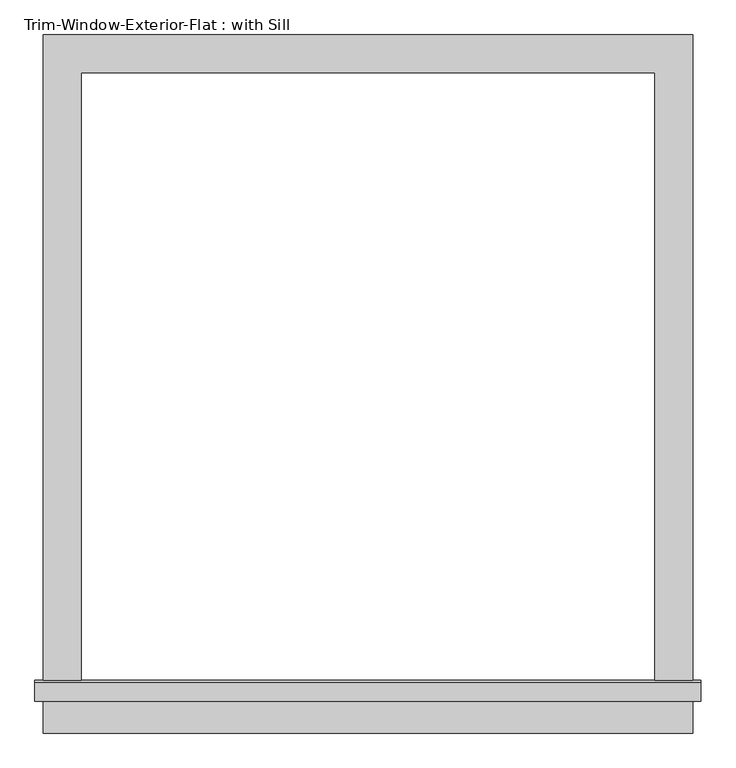
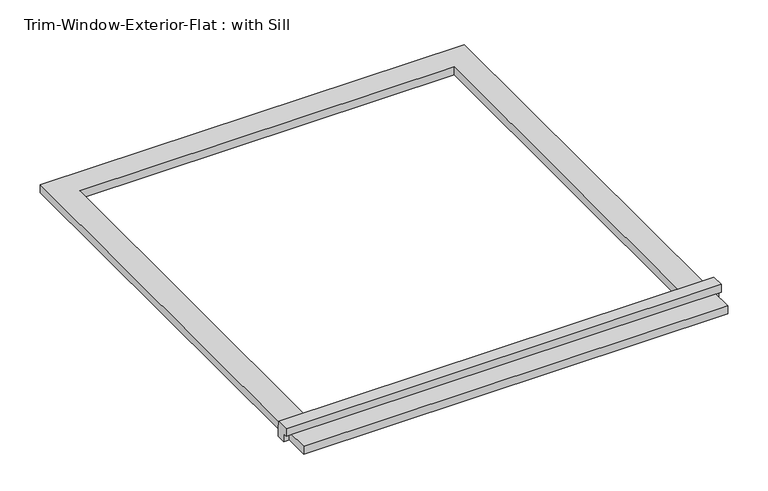
"""IFC4 building model written with IfcOpenShell, lengths in millimetres: proxy geometry, Trim-Window-Exterior-Flat : with Sill."""

from ifc_helpers import new_model, si_unit, frame, origin, origin_with_axes, place, context, project, spatial, polyline, outline, extrude, source, transform, mapped, element, save


def trim_window_exterior_flat_with_sill_41619996(model_context):
    return source(origin(), model_context, "Body", "SweptSolid", [
        extrude(outline(polyline([(488.95, -936.5823709), (488.95, -993.7323709), (-488.95, -993.7323709), (-488.95, -936.5823709), (488.95, -936.5823709)])), origin_with_axes(), (0.0, 0.0, 1.0), 19.05),
        extrude(outline(polyline([(-946.15, 38.1), (-916.8580645, 38.1), (-914.4, 19.05), (-914.4, 0.0), (-936.5823709, 0.0), (-936.5823709, 19.05), (-946.15, 19.05), (-946.15, 38.1)])), frame((-501.65, 0.0, 0.0), z_axis=(1.0, 0.0, 0.0), x_axis=(0.0, 1.0, 0.0)), (0.0, 0.0, 1.0), 1003.3),
        extrude(outline(polyline([(-488.95, 57.15), (488.95, 57.15), (488.95, -914.4), (431.8, -914.4), (431.8, 0.0), (-431.8, 0.0), (-431.8, -914.4), (-488.95, -914.4), (-488.95, 57.15)])), origin_with_axes(), (0.0, 0.0, 1.0), 19.05),
    ])


if __name__ == "__main__":
    model = new_model("IFC4")
    model_context = context("Model", 3, world=origin())
    ifc_project = project(units=[si_unit("LENGTHUNIT", "METRE", prefix="MILLI")], contexts=[model_context])
    site = spatial("IfcSite", under=ifc_project)
    building = spatial("IfcBuilding", under=site)
    placement = place(None, origin())
    trim_window_exterior_flat_with_sill_shape = trim_window_exterior_flat_with_sill_41619996(model_context)
    element("IfcBuildingElementProxy", 1, Name="Trim-Window-Exterior-Flat : with Sill", ObjectType="Trim-Window-Exterior-Flat : with Sill", at=placement, inside=building, context=model_context, shape_type="MappedRepresentation", body=[
        mapped(trim_window_exterior_flat_with_sill_shape, transform((0.0, 0.0, 0.0), x_axis=(1.0, 0.0, 0.0), y_axis=(0.0, 1.0, 0.0), z_axis=(0.0, 0.0, 1.0))),
    ])
    save(model, "model.ifc")

# Revit data of these elements
# Type "Trim-Window-Exterior-Flat : with Sill"
#   Trim Width = 0' - 2 1/4"
#   Trim Thickness_Picture Frame = 0' - 1 1/4"
#   Trim Thickness_with Sill = 0' - 0 3/4"
#   Sill Thickness = 0' - 1 1/4"
#   Opening Width [instance default] = 2' - 0"
#   Opening Height [instance default] = 3' - 0"
#   Default Elevation = 4' - 0"
#   Sill = yes
#   Picture Frame = no
#   Trim Material [instance default] = none
# Element 1 (IfcBuildingElementProxy, "Trim-Window-Exterior-Flat : with Sill")
#   Opening Width = 2' - 10"
#   Trim Material = Clad - White
#   Materials on its faces: "Clad - White"
# Materials
#   "Clad - White": class "Wood", colour RGB 242 242 238, transparency 0, Cost = 0
